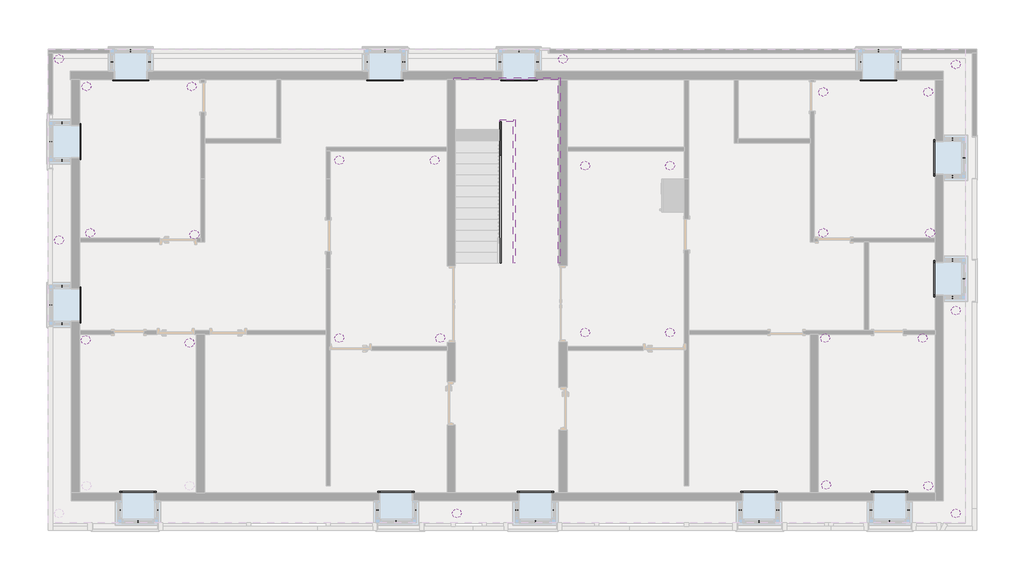
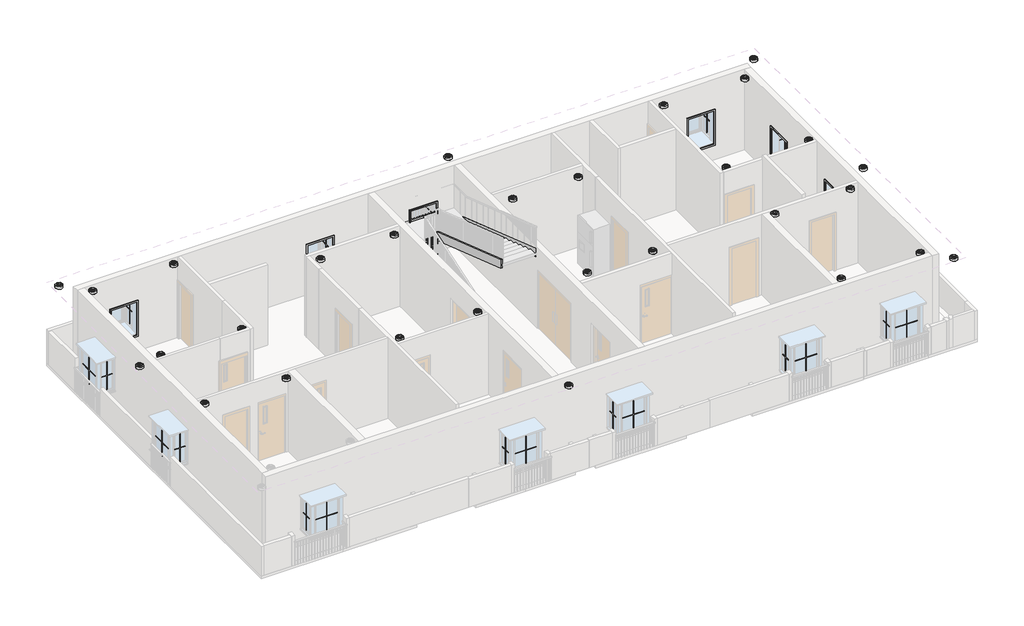
# One storey, part 7 of 7: 52 proxies, 29 light fixtures, 6 members.
"""IFC4 building model written with IfcOpenShell, lengths in millimetres."""

from ifc_helpers import new_model, si_unit, frame, origin, place, context, project, spatial, polyline, outline, extrude, transform, mapped, element, save
from components import muntin_pattern_2x2_muntin_pattern_2x2_95b57395, muntin_pattern_2x2_muntin_pattern_2x2_f03ab90d, trim_window_interior_flat_picture_frame_e50cf7ae, ceiling_light_flat_round_60w_120v_7c4c2a52

model = new_model("IFC4")

# Units and contexts
model_context = context("Model", 3, world=origin())
ifc_project = project(units=[si_unit("LENGTHUNIT", "METRE", prefix="MILLI")], contexts=[model_context])

# Site, building, storey
site = spatial("IfcSite", under=ifc_project)
building = spatial("IfcBuilding", under=site)
storey = spatial("IfcBuildingStorey", under=building, Elevation=3200.4)

# Proxies
placement = place(None, origin())
muntin_pattern_2x2_muntin_pattern_2x2_shape = muntin_pattern_2x2_muntin_pattern_2x2_95b57395(model_context)
element("IfcBuildingElementProxy", 1, Name="Muntin Pattern_2x2 : Muntin Pattern_2x2", ObjectType="Muntin Pattern_2x2 : Muntin Pattern_2x2", at=placement, inside=storey, context=model_context, shape_type="MappedRepresentation", body=[
    mapped(muntin_pattern_2x2_muntin_pattern_2x2_shape, transform((-10814.9987925, 8428.7317329, 3930.65), x_axis=(1.0, 0.0, 0.0), y_axis=(0.0, 1.0, 0.0), z_axis=(0.0, 0.0, 1.0))),
])
element("IfcBuildingElementProxy", 2, Name="Muntin Pattern_2x2 : Muntin Pattern_2x2", ObjectType="Muntin Pattern_2x2 : Muntin Pattern_2x2", at=placement, inside=storey, context=model_context, shape_type="MappedRepresentation", body=[
    mapped(muntin_pattern_2x2_muntin_pattern_2x2_shape, transform((-3791.8987998, 8428.7317329, 3930.65), x_axis=(1.0, 0.0, 0.0), y_axis=(0.0, 1.0, 0.0), z_axis=(0.0, 0.0, 1.0))),
])
element("IfcBuildingElementProxy", 3, Name="Muntin Pattern_2x2 : Muntin Pattern_2x2", ObjectType="Muntin Pattern_2x2 : Muntin Pattern_2x2", at=placement, inside=storey, context=model_context, shape_type="MappedRepresentation", body=[
    mapped(muntin_pattern_2x2_muntin_pattern_2x2_shape, transform((-96.7067989, 8428.7317329, 3930.65), x_axis=(1.0, 0.0, 0.0), y_axis=(0.0, 1.0, 0.0), z_axis=(0.0, 0.0, 1.0))),
])
element("IfcBuildingElementProxy", 4, Name="Muntin Pattern_2x2 : Muntin Pattern_2x2", ObjectType="Muntin Pattern_2x2 : Muntin Pattern_2x2", at=placement, inside=storey, context=model_context, shape_type="MappedRepresentation", body=[
    mapped(muntin_pattern_2x2_muntin_pattern_2x2_shape, transform((9835.2012075, 8428.7317329, 3930.65), x_axis=(1.0, 0.0, 0.0), y_axis=(0.0, 1.0, 0.0), z_axis=(0.0, 0.0, 1.0))),
])
element("IfcBuildingElementProxy", 5, Name="Muntin Pattern_2x2 : Muntin Pattern_2x2", ObjectType="Muntin Pattern_2x2 : Muntin Pattern_2x2", at=placement, inside=storey, context=model_context, shape_type="MappedRepresentation", body=[
    mapped(muntin_pattern_2x2_muntin_pattern_2x2_shape, transform((-10611.7987958, -4582.4182193, 3930.65), x_axis=(-1.0, 0.0, 0.0), y_axis=(0.0, -1.0, 0.0), z_axis=(0.0, 0.0, 1.0))),
])
element("IfcBuildingElementProxy", 6, Name="Muntin Pattern_2x2 : Muntin Pattern_2x2", ObjectType="Muntin Pattern_2x2 : Muntin Pattern_2x2", at=placement, inside=storey, context=model_context, shape_type="MappedRepresentation", body=[
    mapped(muntin_pattern_2x2_muntin_pattern_2x2_shape, transform((-3487.0987998, -4582.4182193, 3930.65), x_axis=(-1.0, 0.0, 0.0), y_axis=(0.0, -1.0, 0.0), z_axis=(0.0, 0.0, 1.0))),
])
element("IfcBuildingElementProxy", 7, Name="Muntin Pattern_2x2 : Muntin Pattern_2x2", ObjectType="Muntin Pattern_2x2 : Muntin Pattern_2x2", at=placement, inside=storey, context=model_context, shape_type="MappedRepresentation", body=[
    mapped(muntin_pattern_2x2_muntin_pattern_2x2_shape, transform((360.4932011, -4582.4182193, 3930.65), x_axis=(-1.0, 0.0, 0.0), y_axis=(0.0, -1.0, 0.0), z_axis=(0.0, 0.0, 1.0))),
])
element("IfcBuildingElementProxy", 8, Name="Muntin Pattern_2x2 : Muntin Pattern_2x2", ObjectType="Muntin Pattern_2x2 : Muntin Pattern_2x2", at=placement, inside=storey, context=model_context, shape_type="MappedRepresentation", body=[
    mapped(muntin_pattern_2x2_muntin_pattern_2x2_shape, transform((6533.2012079, -4582.4182193, 3930.65), x_axis=(-1.0, 0.0, 0.0), y_axis=(0.0, -1.0, 0.0), z_axis=(0.0, 0.0, 1.0))),
])
element("IfcBuildingElementProxy", 9, Name="Muntin Pattern_2x2 : Muntin Pattern_2x2", ObjectType="Muntin Pattern_2x2 : Muntin Pattern_2x2", at=placement, inside=storey, context=model_context, shape_type="MappedRepresentation", body=[
    mapped(muntin_pattern_2x2_muntin_pattern_2x2_shape, transform((10140.0012075, -4582.4182193, 3930.65), x_axis=(-1.0, 0.0, 0.0), y_axis=(0.0, -1.0, 0.0), z_axis=(0.0, 0.0, 1.0))),
])
element("IfcBuildingElementProxy", 10, Name="Muntin Pattern_2x2 : Muntin Pattern_2x2", ObjectType="Muntin Pattern_2x2 : Muntin Pattern_2x2", at=placement, inside=storey, context=model_context, shape_type="MappedRepresentation", body=[
    mapped(muntin_pattern_2x2_muntin_pattern_2x2_shape, transform((12194.2262075, 2126.3567332, 3930.65), x_axis=(0.0, -1.0, 0.0), y_axis=(1.0, 0.0, 0.0), z_axis=(0.0, 0.0, 1.0))),
])
element("IfcBuildingElementProxy", 11, Name="Muntin Pattern_2x2 : Muntin Pattern_2x2", ObjectType="Muntin Pattern_2x2 : Muntin Pattern_2x2", at=placement, inside=storey, context=model_context, shape_type="MappedRepresentation", body=[
    mapped(muntin_pattern_2x2_muntin_pattern_2x2_shape, transform((12194.2262075, 5469.631733, 3930.65), x_axis=(0.0, -1.0, 0.0), y_axis=(1.0, 0.0, 0.0), z_axis=(0.0, 0.0, 1.0))),
])
element("IfcBuildingElementProxy", 12, Name="Muntin Pattern_2x2 : Muntin Pattern_2x2", ObjectType="Muntin Pattern_2x2 : Muntin Pattern_2x2", at=placement, inside=storey, context=model_context, shape_type="MappedRepresentation", body=[
    mapped(muntin_pattern_2x2_muntin_pattern_2x2_shape, transform((-13021.6237925, 1402.4567334, 3930.65), x_axis=(0.0, 1.0, 0.0), y_axis=(-1.0, 0.0, 0.0), z_axis=(0.0, 0.0, 1.0))),
])
element("IfcBuildingElementProxy", 13, Name="Muntin Pattern_2x2 : Muntin Pattern_2x2", ObjectType="Muntin Pattern_2x2 : Muntin Pattern_2x2", at=placement, inside=storey, context=model_context, shape_type="MappedRepresentation", body=[
    mapped(muntin_pattern_2x2_muntin_pattern_2x2_shape, transform((-13021.6237925, 5917.3067329, 3930.65), x_axis=(0.0, 1.0, 0.0), y_axis=(-1.0, 0.0, 0.0), z_axis=(0.0, 0.0, 1.0))),
])
muntin_pattern_2x2_muntin_pattern_2x2_2_shape = muntin_pattern_2x2_muntin_pattern_2x2_f03ab90d(model_context)
element("IfcBuildingElementProxy", 14, Name="Muntin Pattern_2x2 : Muntin Pattern_2x2", ObjectType="Muntin Pattern_2x2 : Muntin Pattern_2x2", at=placement, inside=storey, context=model_context, shape_type="MappedRepresentation", body=[
    mapped(muntin_pattern_2x2_muntin_pattern_2x2_2_shape, transform((-11332.5237925, 8114.4067329, 3930.65), x_axis=(0.0, -1.0, 0.0), y_axis=(1.0, 0.0, 0.0), z_axis=(0.0, 0.0, 1.0))),
])
element("IfcBuildingElementProxy", 15, Name="Muntin Pattern_2x2 : Muntin Pattern_2x2", ObjectType="Muntin Pattern_2x2 : Muntin Pattern_2x2", at=placement, inside=storey, context=model_context, shape_type="MappedRepresentation", body=[
    mapped(muntin_pattern_2x2_muntin_pattern_2x2_2_shape, transform((-10297.4737925, 8114.4067329, 3930.65), x_axis=(0.0, 1.0, 0.0), y_axis=(-1.0, 0.0, 0.0), z_axis=(0.0, 0.0, 1.0))),
])
element("IfcBuildingElementProxy", 16, Name="Muntin Pattern_2x2 : Muntin Pattern_2x2", ObjectType="Muntin Pattern_2x2 : Muntin Pattern_2x2", at=placement, inside=storey, context=model_context, shape_type="MappedRepresentation", body=[
    mapped(muntin_pattern_2x2_muntin_pattern_2x2_2_shape, transform((-4309.4237998, 8114.4067329, 3930.65), x_axis=(0.0, -1.0, 0.0), y_axis=(1.0, 0.0, 0.0), z_axis=(0.0, 0.0, 1.0))),
])
element("IfcBuildingElementProxy", 17, Name="Muntin Pattern_2x2 : Muntin Pattern_2x2", ObjectType="Muntin Pattern_2x2 : Muntin Pattern_2x2", at=placement, inside=storey, context=model_context, shape_type="MappedRepresentation", body=[
    mapped(muntin_pattern_2x2_muntin_pattern_2x2_2_shape, transform((-3274.3737998, 8114.4067329, 3930.65), x_axis=(0.0, 1.0, 0.0), y_axis=(-1.0, 0.0, 0.0), z_axis=(0.0, 0.0, 1.0))),
])
element("IfcBuildingElementProxy", 18, Name="Muntin Pattern_2x2 : Muntin Pattern_2x2", ObjectType="Muntin Pattern_2x2 : Muntin Pattern_2x2", at=placement, inside=storey, context=model_context, shape_type="MappedRepresentation", body=[
    mapped(muntin_pattern_2x2_muntin_pattern_2x2_2_shape, transform((-614.2317989, 8114.4067329, 3930.65), x_axis=(0.0, -1.0, 0.0), y_axis=(1.0, 0.0, 0.0), z_axis=(0.0, 0.0, 1.0))),
])
element("IfcBuildingElementProxy", 19, Name="Muntin Pattern_2x2 : Muntin Pattern_2x2", ObjectType="Muntin Pattern_2x2 : Muntin Pattern_2x2", at=placement, inside=storey, context=model_context, shape_type="MappedRepresentation", body=[
    mapped(muntin_pattern_2x2_muntin_pattern_2x2_2_shape, transform((420.8182011, 8114.4067329, 3930.65), x_axis=(0.0, 1.0, 0.0), y_axis=(-1.0, 0.0, 0.0), z_axis=(0.0, 0.0, 1.0))),
])
element("IfcBuildingElementProxy", 20, Name="Muntin Pattern_2x2 : Muntin Pattern_2x2", ObjectType="Muntin Pattern_2x2 : Muntin Pattern_2x2", at=placement, inside=storey, context=model_context, shape_type="MappedRepresentation", body=[
    mapped(muntin_pattern_2x2_muntin_pattern_2x2_2_shape, transform((9317.6762075, 8114.4067329, 3930.65), x_axis=(0.0, -1.0, 0.0), y_axis=(1.0, 0.0, 0.0), z_axis=(0.0, 0.0, 1.0))),
])
element("IfcBuildingElementProxy", 21, Name="Muntin Pattern_2x2 : Muntin Pattern_2x2", ObjectType="Muntin Pattern_2x2 : Muntin Pattern_2x2", at=placement, inside=storey, context=model_context, shape_type="MappedRepresentation", body=[
    mapped(muntin_pattern_2x2_muntin_pattern_2x2_2_shape, transform((10352.7262075, 8114.4067329, 3930.65), x_axis=(0.0, 1.0, 0.0), y_axis=(-1.0, 0.0, 0.0), z_axis=(0.0, 0.0, 1.0))),
])
element("IfcBuildingElementProxy", 22, Name="Muntin Pattern_2x2 : Muntin Pattern_2x2", ObjectType="Muntin Pattern_2x2 : Muntin Pattern_2x2", at=placement, inside=storey, context=model_context, shape_type="MappedRepresentation", body=[
    mapped(muntin_pattern_2x2_muntin_pattern_2x2_2_shape, transform((-10094.2737958, -4268.0932193, 3930.65), x_axis=(0.0, 1.0, 0.0), y_axis=(-1.0, 0.0, 0.0), z_axis=(0.0, 0.0, 1.0))),
])
element("IfcBuildingElementProxy", 23, Name="Muntin Pattern_2x2 : Muntin Pattern_2x2", ObjectType="Muntin Pattern_2x2 : Muntin Pattern_2x2", at=placement, inside=storey, context=model_context, shape_type="MappedRepresentation", body=[
    mapped(muntin_pattern_2x2_muntin_pattern_2x2_2_shape, transform((-11129.3237958, -4268.0932193, 3930.65), x_axis=(0.0, -1.0, 0.0), y_axis=(1.0, 0.0, 0.0), z_axis=(0.0, 0.0, 1.0))),
])
element("IfcBuildingElementProxy", 24, Name="Muntin Pattern_2x2 : Muntin Pattern_2x2", ObjectType="Muntin Pattern_2x2 : Muntin Pattern_2x2", at=placement, inside=storey, context=model_context, shape_type="MappedRepresentation", body=[
    mapped(muntin_pattern_2x2_muntin_pattern_2x2_2_shape, transform((-2969.5737998, -4268.0932193, 3930.65), x_axis=(0.0, 1.0, 0.0), y_axis=(-1.0, 0.0, 0.0), z_axis=(0.0, 0.0, 1.0))),
])
element("IfcBuildingElementProxy", 25, Name="Muntin Pattern_2x2 : Muntin Pattern_2x2", ObjectType="Muntin Pattern_2x2 : Muntin Pattern_2x2", at=placement, inside=storey, context=model_context, shape_type="MappedRepresentation", body=[
    mapped(muntin_pattern_2x2_muntin_pattern_2x2_2_shape, transform((-4004.6237998, -4268.0932193, 3930.65), x_axis=(0.0, -1.0, 0.0), y_axis=(1.0, 0.0, 0.0), z_axis=(0.0, 0.0, 1.0))),
])
element("IfcBuildingElementProxy", 26, Name="Muntin Pattern_2x2 : Muntin Pattern_2x2", ObjectType="Muntin Pattern_2x2 : Muntin Pattern_2x2", at=placement, inside=storey, context=model_context, shape_type="MappedRepresentation", body=[
    mapped(muntin_pattern_2x2_muntin_pattern_2x2_2_shape, transform((878.0182011, -4268.0932193, 3930.65), x_axis=(0.0, 1.0, 0.0), y_axis=(-1.0, 0.0, 0.0), z_axis=(0.0, 0.0, 1.0))),
])
element("IfcBuildingElementProxy", 27, Name="Muntin Pattern_2x2 : Muntin Pattern_2x2", ObjectType="Muntin Pattern_2x2 : Muntin Pattern_2x2", at=placement, inside=storey, context=model_context, shape_type="MappedRepresentation", body=[
    mapped(muntin_pattern_2x2_muntin_pattern_2x2_2_shape, transform((-157.0317989, -4268.0932193, 3930.65), x_axis=(0.0, -1.0, 0.0), y_axis=(1.0, 0.0, 0.0), z_axis=(0.0, 0.0, 1.0))),
])
element("IfcBuildingElementProxy", 28, Name="Muntin Pattern_2x2 : Muntin Pattern_2x2", ObjectType="Muntin Pattern_2x2 : Muntin Pattern_2x2", at=placement, inside=storey, context=model_context, shape_type="MappedRepresentation", body=[
    mapped(muntin_pattern_2x2_muntin_pattern_2x2_2_shape, transform((7050.7262079, -4268.0932193, 3930.65), x_axis=(0.0, 1.0, 0.0), y_axis=(-1.0, 0.0, 0.0), z_axis=(0.0, 0.0, 1.0))),
])
element("IfcBuildingElementProxy", 29, Name="Muntin Pattern_2x2 : Muntin Pattern_2x2", ObjectType="Muntin Pattern_2x2 : Muntin Pattern_2x2", at=placement, inside=storey, context=model_context, shape_type="MappedRepresentation", body=[
    mapped(muntin_pattern_2x2_muntin_pattern_2x2_2_shape, transform((6015.6762079, -4268.0932193, 3930.65), x_axis=(0.0, -1.0, 0.0), y_axis=(1.0, 0.0, 0.0), z_axis=(0.0, 0.0, 1.0))),
])
element("IfcBuildingElementProxy", 30, Name="Muntin Pattern_2x2 : Muntin Pattern_2x2", ObjectType="Muntin Pattern_2x2 : Muntin Pattern_2x2", at=placement, inside=storey, context=model_context, shape_type="MappedRepresentation", body=[
    mapped(muntin_pattern_2x2_muntin_pattern_2x2_2_shape, transform((10657.5262075, -4268.0932193, 3930.65), x_axis=(0.0, 1.0, 0.0), y_axis=(-1.0, 0.0, 0.0), z_axis=(0.0, 0.0, 1.0))),
])
element("IfcBuildingElementProxy", 31, Name="Muntin Pattern_2x2 : Muntin Pattern_2x2", ObjectType="Muntin Pattern_2x2 : Muntin Pattern_2x2", at=placement, inside=storey, context=model_context, shape_type="MappedRepresentation", body=[
    mapped(muntin_pattern_2x2_muntin_pattern_2x2_2_shape, transform((9622.4762075, -4268.0932193, 3930.65), x_axis=(0.0, -1.0, 0.0), y_axis=(1.0, 0.0, 0.0), z_axis=(0.0, 0.0, 1.0))),
])
element("IfcBuildingElementProxy", 32, Name="Muntin Pattern_2x2 : Muntin Pattern_2x2", ObjectType="Muntin Pattern_2x2 : Muntin Pattern_2x2", at=placement, inside=storey, context=model_context, shape_type="MappedRepresentation", body=[
    mapped(muntin_pattern_2x2_muntin_pattern_2x2_2_shape, transform((11879.9012075, 2643.8817332, 3930.65), x_axis=(-1.0, 0.0, 0.0), y_axis=(0.0, -1.0, 0.0), z_axis=(0.0, 0.0, 1.0))),
])
element("IfcBuildingElementProxy", 33, Name="Muntin Pattern_2x2 : Muntin Pattern_2x2", ObjectType="Muntin Pattern_2x2 : Muntin Pattern_2x2", at=placement, inside=storey, context=model_context, shape_type="MappedRepresentation", body=[
    mapped(muntin_pattern_2x2_muntin_pattern_2x2_2_shape, transform((11879.9012075, 1608.8317332, 3930.65), x_axis=(1.0, 0.0, 0.0), y_axis=(0.0, 1.0, 0.0), z_axis=(0.0, 0.0, 1.0))),
])
element("IfcBuildingElementProxy", 34, Name="Muntin Pattern_2x2 : Muntin Pattern_2x2", ObjectType="Muntin Pattern_2x2 : Muntin Pattern_2x2", at=placement, inside=storey, context=model_context, shape_type="MappedRepresentation", body=[
    mapped(muntin_pattern_2x2_muntin_pattern_2x2_2_shape, transform((11879.9012075, 5987.156733, 3930.65), x_axis=(-1.0, 0.0, 0.0), y_axis=(0.0, -1.0, 0.0), z_axis=(0.0, 0.0, 1.0))),
])
element("IfcBuildingElementProxy", 35, Name="Muntin Pattern_2x2 : Muntin Pattern_2x2", ObjectType="Muntin Pattern_2x2 : Muntin Pattern_2x2", at=placement, inside=storey, context=model_context, shape_type="MappedRepresentation", body=[
    mapped(muntin_pattern_2x2_muntin_pattern_2x2_2_shape, transform((11879.9012075, 4952.106733, 3930.65), x_axis=(1.0, 0.0, 0.0), y_axis=(0.0, 1.0, 0.0), z_axis=(0.0, 0.0, 1.0))),
])
element("IfcBuildingElementProxy", 36, Name="Muntin Pattern_2x2 : Muntin Pattern_2x2", ObjectType="Muntin Pattern_2x2 : Muntin Pattern_2x2", at=placement, inside=storey, context=model_context, shape_type="MappedRepresentation", body=[
    mapped(muntin_pattern_2x2_muntin_pattern_2x2_2_shape, transform((-12707.2987925, 884.9317334, 3930.65), x_axis=(1.0, 0.0, 0.0), y_axis=(0.0, 1.0, 0.0), z_axis=(0.0, 0.0, 1.0))),
])
element("IfcBuildingElementProxy", 37, Name="Muntin Pattern_2x2 : Muntin Pattern_2x2", ObjectType="Muntin Pattern_2x2 : Muntin Pattern_2x2", at=placement, inside=storey, context=model_context, shape_type="MappedRepresentation", body=[
    mapped(muntin_pattern_2x2_muntin_pattern_2x2_2_shape, transform((-12707.2987925, 1919.9817334, 3930.65), x_axis=(-1.0, 0.0, 0.0), y_axis=(0.0, -1.0, 0.0), z_axis=(0.0, 0.0, 1.0))),
])
element("IfcBuildingElementProxy", 38, Name="Muntin Pattern_2x2 : Muntin Pattern_2x2", ObjectType="Muntin Pattern_2x2 : Muntin Pattern_2x2", at=placement, inside=storey, context=model_context, shape_type="MappedRepresentation", body=[
    mapped(muntin_pattern_2x2_muntin_pattern_2x2_2_shape, transform((-12707.2987925, 5399.7817329, 3930.65), x_axis=(1.0, 0.0, 0.0), y_axis=(0.0, 1.0, 0.0), z_axis=(0.0, 0.0, 1.0))),
])
element("IfcBuildingElementProxy", 39, Name="Muntin Pattern_2x2 : Muntin Pattern_2x2", ObjectType="Muntin Pattern_2x2 : Muntin Pattern_2x2", at=placement, inside=storey, context=model_context, shape_type="MappedRepresentation", body=[
    mapped(muntin_pattern_2x2_muntin_pattern_2x2_2_shape, transform((-12707.2987925, 6434.8317329, 3930.65), x_axis=(-1.0, 0.0, 0.0), y_axis=(0.0, -1.0, 0.0), z_axis=(0.0, 0.0, 1.0))),
])
trim_window_interior_flat_picture_frame_shape = trim_window_interior_flat_picture_frame_e50cf7ae(model_context)
element("IfcBuildingElementProxy", 40, Name="Trim-Window-Interior-Flat : Picture Frame", ObjectType="Trim-Window-Interior-Flat : Picture Frame", at=placement, inside=storey, context=model_context, shape_type="MappedRepresentation", body=[
    mapped(trim_window_interior_flat_picture_frame_shape, transform((-10814.9987925, 7631.8067329, 5080.0), x_axis=(1.0, 0.0, 0.0), y_axis=(0.0, 0.0, 1.0), z_axis=(0.0, -1.0, 0.0))),
])
element("IfcBuildingElementProxy", 41, Name="Trim-Window-Interior-Flat : Picture Frame", ObjectType="Trim-Window-Interior-Flat : Picture Frame", at=placement, inside=storey, context=model_context, shape_type="MappedRepresentation", body=[
    mapped(trim_window_interior_flat_picture_frame_shape, transform((-3791.8987998, 7631.8067329, 5080.0), x_axis=(1.0, 0.0, 0.0), y_axis=(0.0, 0.0, 1.0), z_axis=(0.0, -1.0, 0.0))),
])
element("IfcBuildingElementProxy", 42, Name="Trim-Window-Interior-Flat : Picture Frame", ObjectType="Trim-Window-Interior-Flat : Picture Frame", at=placement, inside=storey, context=model_context, shape_type="MappedRepresentation", body=[
    mapped(trim_window_interior_flat_picture_frame_shape, transform((-96.7067989, 7631.8067329, 5080.0), x_axis=(1.0, 0.0, 0.0), y_axis=(0.0, 0.0, 1.0), z_axis=(0.0, -1.0, 0.0))),
])
element("IfcBuildingElementProxy", 43, Name="Trim-Window-Interior-Flat : Picture Frame", ObjectType="Trim-Window-Interior-Flat : Picture Frame", at=placement, inside=storey, context=model_context, shape_type="MappedRepresentation", body=[
    mapped(trim_window_interior_flat_picture_frame_shape, transform((9835.2012075, 7631.8067329, 5080.0), x_axis=(1.0, 0.0, 0.0), y_axis=(0.0, 0.0, 1.0), z_axis=(0.0, -1.0, 0.0))),
])
element("IfcBuildingElementProxy", 44, Name="Trim-Window-Interior-Flat : Picture Frame", ObjectType="Trim-Window-Interior-Flat : Picture Frame", at=placement, inside=storey, context=model_context, shape_type="MappedRepresentation", body=[
    mapped(trim_window_interior_flat_picture_frame_shape, transform((-10611.7987958, -3785.4932193, 5080.0), x_axis=(-1.0, 0.0, 0.0), y_axis=(0.0, 0.0, 1.0), z_axis=(0.0, 1.0, 0.0))),
])
element("IfcBuildingElementProxy", 45, Name="Trim-Window-Interior-Flat : Picture Frame", ObjectType="Trim-Window-Interior-Flat : Picture Frame", at=placement, inside=storey, context=model_context, shape_type="MappedRepresentation", body=[
    mapped(trim_window_interior_flat_picture_frame_shape, transform((-3487.0987998, -3785.4932193, 5080.0), x_axis=(-1.0, 0.0, 0.0), y_axis=(0.0, 0.0, 1.0), z_axis=(0.0, 1.0, 0.0))),
])
element("IfcBuildingElementProxy", 46, Name="Trim-Window-Interior-Flat : Picture Frame", ObjectType="Trim-Window-Interior-Flat : Picture Frame", at=placement, inside=storey, context=model_context, shape_type="MappedRepresentation", body=[
    mapped(trim_window_interior_flat_picture_frame_shape, transform((360.4932011, -3785.4932193, 5080.0), x_axis=(-1.0, 0.0, 0.0), y_axis=(0.0, 0.0, 1.0), z_axis=(0.0, 1.0, 0.0))),
])
element("IfcBuildingElementProxy", 47, Name="Trim-Window-Interior-Flat : Picture Frame", ObjectType="Trim-Window-Interior-Flat : Picture Frame", at=placement, inside=storey, context=model_context, shape_type="MappedRepresentation", body=[
    mapped(trim_window_interior_flat_picture_frame_shape, transform((6533.2012079, -3785.4932193, 5080.0), x_axis=(-1.0, 0.0, 0.0), y_axis=(0.0, 0.0, 1.0), z_axis=(0.0, 1.0, 0.0))),
])
element("IfcBuildingElementProxy", 48, Name="Trim-Window-Interior-Flat : Picture Frame", ObjectType="Trim-Window-Interior-Flat : Picture Frame", at=placement, inside=storey, context=model_context, shape_type="MappedRepresentation", body=[
    mapped(trim_window_interior_flat_picture_frame_shape, transform((10140.0012075, -3785.4932193, 5080.0), x_axis=(-1.0, 0.0, 0.0), y_axis=(0.0, 0.0, 1.0), z_axis=(0.0, 1.0, 0.0))),
])
element("IfcBuildingElementProxy", 49, Name="Trim-Window-Interior-Flat : Picture Frame", ObjectType="Trim-Window-Interior-Flat : Picture Frame", at=placement, inside=storey, context=model_context, shape_type="MappedRepresentation", body=[
    mapped(trim_window_interior_flat_picture_frame_shape, transform((11397.3012075, 2126.3567332, 5080.0), x_axis=(0.0, -1.0, 0.0), y_axis=(0.0, 0.0, 1.0), z_axis=(-1.0, 0.0, 0.0))),
])
element("IfcBuildingElementProxy", 50, Name="Trim-Window-Interior-Flat : Picture Frame", ObjectType="Trim-Window-Interior-Flat : Picture Frame", at=placement, inside=storey, context=model_context, shape_type="MappedRepresentation", body=[
    mapped(trim_window_interior_flat_picture_frame_shape, transform((11397.3012075, 5469.631733, 5080.0), x_axis=(0.0, -1.0, 0.0), y_axis=(0.0, 0.0, 1.0), z_axis=(-1.0, 0.0, 0.0))),
])
element("IfcBuildingElementProxy", 51, Name="Trim-Window-Interior-Flat : Picture Frame", ObjectType="Trim-Window-Interior-Flat : Picture Frame", at=placement, inside=storey, context=model_context, shape_type="MappedRepresentation", body=[
    mapped(trim_window_interior_flat_picture_frame_shape, transform((-12224.6987925, 1402.4567334, 5080.0), x_axis=(0.0, 1.0, 0.0), y_axis=(0.0, 0.0, 1.0), z_axis=(1.0, 0.0, 0.0))),
])
element("IfcBuildingElementProxy", 52, Name="Trim-Window-Interior-Flat : Picture Frame", ObjectType="Trim-Window-Interior-Flat : Picture Frame", at=placement, inside=storey, context=model_context, shape_type="MappedRepresentation", body=[
    mapped(trim_window_interior_flat_picture_frame_shape, transform((-12224.6987925, 5917.3067329, 5080.0), x_axis=(0.0, 1.0, 0.0), y_axis=(0.0, 0.0, 1.0), z_axis=(1.0, 0.0, 0.0))),
])

# Light fixtures
ceiling_light_flat_round_60w_120v_shape = ceiling_light_flat_round_60w_120v_7c4c2a52(model_context)
element("IfcLightFixture", 53, ObjectType="Ceiling Light - Flat Round : 60W - 120V", at=placement, inside=storey, context=model_context, shape_type="MappedRepresentation", body=[
    mapped(ceiling_light_flat_round_60w_120v_shape, transform((-12796.1987925, 8203.3067329, 3810.0), x_axis=(1.0, 0.0, 0.0), y_axis=(0.0, 1.0, 0.0), z_axis=(0.0, 0.0, 1.0))),
])
element("IfcLightFixture", 54, ObjectType="Ceiling Light - Flat Round : 60W - 120V", at=placement, inside=storey, context=model_context, shape_type="MappedRepresentation", body=[
    mapped(ceiling_light_flat_round_60w_120v_shape, transform((-12796.1987925, 3193.1567332, 3810.0), x_axis=(1.0, 0.0, 0.0), y_axis=(0.0, 1.0, 0.0), z_axis=(0.0, 0.0, 1.0))),
])
element("IfcLightFixture", 55, ObjectType="Ceiling Light - Flat Round : 60W - 120V", at=placement, inside=storey, context=model_context, shape_type="MappedRepresentation", body=[
    mapped(ceiling_light_flat_round_60w_120v_shape, transform((-1810.6987998, -4356.9932193, 3810.0), x_axis=(1.0, 0.0, 0.0), y_axis=(0.0, 1.0, 0.0), z_axis=(0.0, 0.0, 1.0))),
])
element("IfcLightFixture", 56, ObjectType="Ceiling Light - Flat Round : 60W - 120V", at=placement, inside=storey, context=model_context, shape_type="MappedRepresentation", body=[
    mapped(ceiling_light_flat_round_60w_120v_shape, transform((11968.8012075, -4356.9932193, 3810.0), x_axis=(1.0, 0.0, 0.0), y_axis=(0.0, 1.0, 0.0), z_axis=(0.0, 0.0, 1.0))),
])
element("IfcLightFixture", 57, ObjectType="Ceiling Light - Flat Round : 60W - 120V", at=placement, inside=storey, context=model_context, shape_type="MappedRepresentation", body=[
    mapped(ceiling_light_flat_round_60w_120v_shape, transform((11968.8012075, 1250.0567334, 3810.0), x_axis=(1.0, 0.0, 0.0), y_axis=(0.0, 1.0, 0.0), z_axis=(0.0, 0.0, 1.0))),
])
element("IfcLightFixture", 58, ObjectType="Ceiling Light - Flat Round : 60W - 120V", at=placement, inside=storey, context=model_context, shape_type="MappedRepresentation", body=[
    mapped(ceiling_light_flat_round_60w_120v_shape, transform((11968.8012075, 8050.9067329, 3810.0), x_axis=(1.0, 0.0, 0.0), y_axis=(0.0, 1.0, 0.0), z_axis=(0.0, 0.0, 1.0))),
])
element("IfcLightFixture", 59, ObjectType="Ceiling Light - Flat Round : 60W - 120V", at=placement, inside=storey, context=model_context, shape_type="MappedRepresentation", body=[
    mapped(ceiling_light_flat_round_60w_120v_shape, transform((1122.4932011, 8203.3067329, 3810.0), x_axis=(1.0, 0.0, 0.0), y_axis=(0.0, 1.0, 0.0), z_axis=(0.0, 0.0, 1.0))),
])
element("IfcLightFixture", 60, ObjectType="Ceiling Light - Flat Round : 60W - 120V", at=placement, inside=storey, context=model_context, shape_type="MappedRepresentation", body=[
    mapped(ceiling_light_flat_round_60w_120v_shape, transform((-9189.3987992, 357.6578621, 3810.0), x_axis=(1.0, 0.0, 0.0), y_axis=(0.0, 1.0, 0.0), z_axis=(0.0, 0.0, 1.0))),
])
element("IfcLightFixture", 61, ObjectType="Ceiling Light - Flat Round : 60W - 120V", at=placement, inside=storey, context=model_context, shape_type="MappedRepresentation", body=[
    mapped(ceiling_light_flat_round_60w_120v_shape, transform((-12059.5987925, 437.2567334, 3810.0), x_axis=(1.0, 0.0, 0.0), y_axis=(0.0, 1.0, 0.0), z_axis=(0.0, 0.0, 1.0))),
])
element("IfcLightFixture", 62, ObjectType="Ceiling Light - Flat Round : 60W - 120V", at=placement, inside=storey, context=model_context, shape_type="MappedRepresentation", body=[
    mapped(ceiling_light_flat_round_60w_120v_shape, transform((-12034.1987925, 7441.3067329, 3810.0), x_axis=(1.0, 0.0, 0.0), y_axis=(0.0, 1.0, 0.0), z_axis=(0.0, 0.0, 1.0))),
])
element("IfcLightFixture", 63, ObjectType="Ceiling Light - Flat Round : 60W - 120V", at=placement, inside=storey, context=model_context, shape_type="MappedRepresentation", body=[
    mapped(ceiling_light_flat_round_60w_120v_shape, transform((-9132.2487992, 7441.3067329, 3810.0), x_axis=(1.0, 0.0, 0.0), y_axis=(0.0, 1.0, 0.0), z_axis=(0.0, 0.0, 1.0))),
])
element("IfcLightFixture", 64, ObjectType="Ceiling Light - Flat Round : 60W - 120V", at=placement, inside=storey, context=model_context, shape_type="MappedRepresentation", body=[
    mapped(ceiling_light_flat_round_60w_120v_shape, transform((-11932.5987925, 3396.3567332, 3810.0), x_axis=(1.0, 0.0, 0.0), y_axis=(0.0, 1.0, 0.0), z_axis=(0.0, 0.0, 1.0))),
])
element("IfcLightFixture", 65, ObjectType="Ceiling Light - Flat Round : 60W - 120V", at=placement, inside=storey, context=model_context, shape_type="MappedRepresentation", body=[
    mapped(ceiling_light_flat_round_60w_120v_shape, transform((-9056.0487992, 3345.5567332, 3810.0), x_axis=(1.0, 0.0, 0.0), y_axis=(0.0, 1.0, 0.0), z_axis=(0.0, 0.0, 1.0))),
])
element("IfcLightFixture", 66, ObjectType="Ceiling Light - Flat Round : 60W - 120V", at=placement, inside=storey, context=model_context, shape_type="MappedRepresentation", body=[
    mapped(ceiling_light_flat_round_60w_120v_shape, transform((8304.8512079, 7288.9067329, 3810.0), x_axis=(1.0, 0.0, 0.0), y_axis=(0.0, 1.0, 0.0), z_axis=(0.0, 0.0, 1.0))),
])
element("IfcLightFixture", 67, ObjectType="Ceiling Light - Flat Round : 60W - 120V", at=placement, inside=storey, context=model_context, shape_type="MappedRepresentation", body=[
    mapped(ceiling_light_flat_round_60w_120v_shape, transform((11206.8012075, 7288.9067329, 3810.0), x_axis=(1.0, 0.0, 0.0), y_axis=(0.0, 1.0, 0.0), z_axis=(0.0, 0.0, 1.0))),
])
element("IfcLightFixture", 68, ObjectType="Ceiling Light - Flat Round : 60W - 120V", at=placement, inside=storey, context=model_context, shape_type="MappedRepresentation", body=[
    mapped(ceiling_light_flat_round_60w_120v_shape, transform((8304.8512079, 3396.3567332, 3810.0), x_axis=(1.0, 0.0, 0.0), y_axis=(0.0, 1.0, 0.0), z_axis=(0.0, 0.0, 1.0))),
])
element("IfcLightFixture", 69, ObjectType="Ceiling Light - Flat Round : 60W - 120V", at=placement, inside=storey, context=model_context, shape_type="MappedRepresentation", body=[
    mapped(ceiling_light_flat_round_60w_120v_shape, transform((11257.6012075, 3396.3567332, 3810.0), x_axis=(1.0, 0.0, 0.0), y_axis=(0.0, 1.0, 0.0), z_axis=(0.0, 0.0, 1.0))),
])
element("IfcLightFixture", 70, ObjectType="Ceiling Light - Flat Round : 60W - 120V", at=placement, inside=storey, context=model_context, shape_type="MappedRepresentation", body=[
    mapped(ceiling_light_flat_round_60w_120v_shape, transform((8362.0012079, 488.0567334, 3810.0), x_axis=(1.0, 0.0, 0.0), y_axis=(0.0, 1.0, 0.0), z_axis=(0.0, 0.0, 1.0))),
])
element("IfcLightFixture", 71, ObjectType="Ceiling Light - Flat Round : 60W - 120V", at=placement, inside=storey, context=model_context, shape_type="MappedRepresentation", body=[
    mapped(ceiling_light_flat_round_60w_120v_shape, transform((11054.4012075, 488.0567334, 3810.0), x_axis=(1.0, 0.0, 0.0), y_axis=(0.0, 1.0, 0.0), z_axis=(0.0, 0.0, 1.0))),
])
element("IfcLightFixture", 72, ObjectType="Ceiling Light - Flat Round : 60W - 120V", at=placement, inside=storey, context=model_context, shape_type="MappedRepresentation", body=[
    mapped(ceiling_light_flat_round_60w_120v_shape, transform((8387.4012079, -3569.5932193, 3810.0), x_axis=(1.0, 0.0, 0.0), y_axis=(0.0, 1.0, 0.0), z_axis=(0.0, 0.0, 1.0))),
])
element("IfcLightFixture", 73, ObjectType="Ceiling Light - Flat Round : 60W - 120V", at=placement, inside=storey, context=model_context, shape_type="MappedRepresentation", body=[
    mapped(ceiling_light_flat_round_60w_120v_shape, transform((11206.8012075, -3594.9932193, 3810.0), x_axis=(1.0, 0.0, 0.0), y_axis=(0.0, 1.0, 0.0), z_axis=(0.0, 0.0, 1.0))),
])
element("IfcLightFixture", 74, ObjectType="Ceiling Light - Flat Round : 60W - 120V", at=placement, inside=storey, context=model_context, shape_type="MappedRepresentation", body=[
    mapped(ceiling_light_flat_round_60w_120v_shape, transform((-2420.2987998, 5402.9567329, 3810.0), x_axis=(1.0, 0.0, 0.0), y_axis=(0.0, 1.0, 0.0), z_axis=(0.0, 0.0, 1.0))),
])
element("IfcLightFixture", 75, ObjectType="Ceiling Light - Flat Round : 60W - 120V", at=placement, inside=storey, context=model_context, shape_type="MappedRepresentation", body=[
    mapped(ceiling_light_flat_round_60w_120v_shape, transform((1732.0932011, 5250.5567329, 3810.0), x_axis=(1.0, 0.0, 0.0), y_axis=(0.0, 1.0, 0.0), z_axis=(0.0, 0.0, 1.0))),
])
element("IfcLightFixture", 76, ObjectType="Ceiling Light - Flat Round : 60W - 120V", at=placement, inside=storey, context=model_context, shape_type="MappedRepresentation", body=[
    mapped(ceiling_light_flat_round_60w_120v_shape, transform((4075.7512082, 5250.5567329, 3810.0), x_axis=(1.0, 0.0, 0.0), y_axis=(0.0, 1.0, 0.0), z_axis=(0.0, 0.0, 1.0))),
])
element("IfcLightFixture", 77, ObjectType="Ceiling Light - Flat Round : 60W - 120V", at=placement, inside=storey, context=model_context, shape_type="MappedRepresentation", body=[
    mapped(ceiling_light_flat_round_60w_120v_shape, transform((1732.0932011, 640.4567334, 3810.0), x_axis=(1.0, 0.0, 0.0), y_axis=(0.0, 1.0, 0.0), z_axis=(0.0, 0.0, 1.0))),
])
element("IfcLightFixture", 78, ObjectType="Ceiling Light - Flat Round : 60W - 120V", at=placement, inside=storey, context=model_context, shape_type="MappedRepresentation", body=[
    mapped(ceiling_light_flat_round_60w_120v_shape, transform((4075.7512082, 640.4567334, 3810.0), x_axis=(1.0, 0.0, 0.0), y_axis=(0.0, 1.0, 0.0), z_axis=(0.0, 0.0, 1.0))),
])
element("IfcLightFixture", 79, ObjectType="Ceiling Light - Flat Round : 60W - 120V", at=placement, inside=storey, context=model_context, shape_type="MappedRepresentation", body=[
    mapped(ceiling_light_flat_round_60w_120v_shape, transform((-5055.5487995, 5402.9567329, 3810.0), x_axis=(1.0, 0.0, 0.0), y_axis=(0.0, 1.0, 0.0), z_axis=(0.0, 0.0, 1.0))),
])
element("IfcLightFixture", 80, ObjectType="Ceiling Light - Flat Round : 60W - 120V", at=placement, inside=storey, context=model_context, shape_type="MappedRepresentation", body=[
    mapped(ceiling_light_flat_round_60w_120v_shape, transform((-5055.5487995, 488.0567334, 3810.0), x_axis=(1.0, 0.0, 0.0), y_axis=(0.0, 1.0, 0.0), z_axis=(0.0, 0.0, 1.0))),
])
element("IfcLightFixture", 81, ObjectType="Ceiling Light - Flat Round : 60W - 120V", at=placement, inside=storey, context=model_context, shape_type="MappedRepresentation", body=[
    mapped(ceiling_light_flat_round_60w_120v_shape, transform((-2267.8987998, 488.0567334, 3810.0), x_axis=(1.0, 0.0, 0.0), y_axis=(0.0, 1.0, 0.0), z_axis=(0.0, 0.0, 1.0))),
])

# Members
element("IfcMember", 82, ObjectType="Stringer - 2\" Width", at=placement, inside=storey, context=model_context, shape_type="SweptSolid", body=[
    extrude(outline(polyline([(2564.5067329, 3200.4), (2564.5067329, 3393.638056), (6486.7524627, 4724.4), (7435.4093802, 4724.4), (2943.6199065, 3200.4), (2564.5067329, 3200.4)])), frame((-1899.5987998, 0.0, 0.0), z_axis=(1.0, 0.0, 0.0), x_axis=(0.0, 1.0, 0.0)), (0.0, 0.0, 1.0), 50.8),
])
element("IfcMember", 83, ObjectType="Stringer - 2\" Width", at=placement, inside=storey, context=model_context, shape_type="SweptSolid", body=[
    extrude(outline(polyline([(-1899.5987998, 7631.8067329), (-1899.5987998, 7682.6067329), (996.0012002, 7682.6067329), (996.0012002, 7631.8067329), (-1899.5987998, 7631.8067329)])), frame((0.0, 0.0, 4419.6), z_axis=(0.0, 0.0, 1.0), x_axis=(1.0, 0.0, 0.0)), (0.0, 0.0, 1.0), 304.8),
])
element("IfcMember", 84, ObjectType="Stringer - 2\" Width", at=placement, inside=storey, context=model_context, shape_type="SweptSolid", body=[
    extrude(outline(polyline([(7682.6067329, 4449.325556), (7682.6067329, 4419.6), (6821.5619804, 4419.6), (2564.5067329, 5863.9580304), (2564.5067329, 6185.8237702), (7682.6067329, 4449.325556)])), frame((996.0012002, 0.0, 0.0), z_axis=(1.0, 0.0, 0.0), x_axis=(0.0, 1.0, 0.0)), (0.0, 0.0, 1.0), 50.8),
])
element("IfcMember", 85, ObjectType="Stringer - 2\" Width", at=placement, inside=storey, context=model_context, shape_type="SweptSolid", body=[
    extrude(outline(polyline([(2564.5067329, 3200.4), (2564.5067329, 3393.638056), (6476.1067329, 4720.788056), (6476.1067329, 4398.9223161), (2943.6199065, 3200.4), (2564.5067329, 3200.4)])), frame((-629.5987998, 0.0, 0.0), z_axis=(1.0, 0.0, 0.0), x_axis=(0.0, 1.0, 0.0)), (0.0, 0.0, 1.0), 50.8),
])
element("IfcMember", 86, ObjectType="Stringer - 2\" Width", at=placement, inside=storey, context=model_context, shape_type="SweptSolid", body=[
    extrude(outline(polyline([(-629.5987998, 6476.1067329), (-629.5987998, 6526.9067329), (-248.5987915, 6526.9067329), (-248.5987915, 6476.1067329), (-629.5987998, 6476.1067329)])), frame((0.0, 0.0, 4419.6), z_axis=(0.0, 0.0, 1.0), x_axis=(1.0, 0.0, 0.0)), (0.0, 0.0, 1.0), 304.8),
])
element("IfcMember", 87, ObjectType="Stringer - 2\" Width", at=placement, inside=storey, context=model_context, shape_type="SweptSolid", body=[
    extrude(outline(polyline([(6526.9067329, 4841.438056), (6526.9067329, 4519.5723161), (2564.5067329, 5863.9580304), (2564.5067329, 6185.8237702), (6526.9067329, 4841.438056)])), frame((-248.5987915, 0.0, 0.0), z_axis=(1.0, 0.0, 0.0), x_axis=(0.0, 1.0, 0.0)), (0.0, 0.0, 1.0), 50.8),
])

save(model, "model.ifc")

# Revit data of these elements
# Type "Muntin Pattern_2x2 : Muntin Pattern_2x2"
#   Width [instance default] = 4' - 0"
#   Thickness = 0' - 0 1/2"
#   Height [instance default] = 4' - 0"
#   Distance = 0' - 0 3/4"
#   Interior Material [instance default] = none
#   Exterior Material [instance default] = none
#   Default Elevation = 0
# Type "Trim-Window-Interior-Flat : Picture Frame"
#   Trim Thickness_Picture Frame = 0' - 1 1/4"
#   Trim Width = 0' - 2 1/4"
#   Trim Thickness_with Sill = 0' - 0 3/4"
#   Sill Thickness = 0' - 1 1/4"
#   Opening Width [instance default] = 2' - 0"
#   Opening Height [instance default] = 3' - 0"
#   Default Elevation = 4' - 0"
#   Sill = no
#   Picture Frame = yes
#   Trim Material [instance default] = none
# Type "Ceiling Light - Flat Round : 60W - 120V"
#   Lamp = "A-19"
#   Assembly Code = "D5020220"
#   Wattage = 60 W
#   built-in parameter 1150110 = 1 (stored number, unit not read)
#   built-in parameter 1114217 = 1 (stored number, unit not read)
#   built-in parameter 1150109 = 1 (stored number, unit not read)
#   built-in parameter 1150113 = 1 (stored number, unit not read)
#   built-in parameter 1150115 = 1 (stored number, unit not read)
#   built-in parameter 1150105 = 272.155 (stored number, unit not read)
#   Light Source Symbol Size = 2' - 0"
#   built-in parameter 1150112 = 1 (stored number, unit not read)
#   built-in parameter 1150114 = 1 (stored number, unit not read)
#   built-in parameter 1150107 = 2800 (stored number, unit not read)
#   built-in parameter 1150106 = 2.72155 (stored number, unit not read)
#   Emit from Circle Diameter = 0' - 10"
#   built-in parameter 1150104 = 1.32387 (stored number, unit not read)
#   Ballast Voltage = 120 V
#   built-in parameter 1114218 = 1 (stored number, unit not read)
#   built-in parameter 1150133 = 10 (stored number, unit not read)
#   Lumens = 855 lm
#   Apparent Load = 60 VA
#   built-in parameter 1150134 = 4
#   built-in parameter 1150137 = 1
#   Color Filter = 16777215
#   built-in parameter 1140040 [instance default] = 1
#   Ballast Number of Poles = 1
#   Light Box Material = Steel, Paint Finish, Dark Gray, Matte
#   Diffuser Material = Glass, White, High Luminance
#   Wattage Comments = ""
#   Emit Shape Visible in Rendering = no
#   Dimming Lamp Color Temperature Shift = (empty or 0)
#   Default Elevation = 0
# Elements 1, 2, 3, 4, 5, 6, 7, 8, 9, 10, 11, 12, 13 (IfcBuildingElementProxy, "Muntin Pattern_2x2 : Muntin Pattern_2x2")
#   Width = 2' - 6 1/2"
#   Height = 3' - 6 1/2"
#   Interior Material = Wood - Stained
#   Exterior Material = Clad - White
#   Phase Created = New Construction
#   Materials on its faces: "Clad - White", "Wood - Stained"
# Elements 14, 15, 16, 17, 18, 19, 20, 21, 22, 23, 24, 25, 26, 27, 28, 29, 30, 31, 32, 33, 34, 35, 36, 37, 38, 39 (IfcBuildingElementProxy, "Muntin Pattern_2x2 : Muntin Pattern_2x2")
#   Width = 1' - 2 1/2"
#   Height = 3' - 6 1/2"
#   Interior Material = Wood - Stained
#   Exterior Material = Clad - White
#   Phase Created = New Construction
#   Materials on its faces: "Clad - White", "Wood - Stained"
# Elements 40, 41, 42, 43, 44, 45, 46, 47, 48, 49, 50, 51, 52 (IfcBuildingElementProxy, "Trim-Window-Interior-Flat : Picture Frame")
#   Opening Width = 3' - 0"
#   Opening Height = 4' - 2"
#   Trim Material = Wood - Stained
#   Phase Created = New Construction
#   Materials on its faces: "Wood - Stained"
# Element 53 (IfcLightFixture, "Ceiling Light - Flat Round : 60W - 120V")
#   Mark = "28"
#   built-in parameter 1140040 = 1
#   Phase Created = New Construction
#   Materials on its faces: "Glass, White, High Luminance", "Steel, Paint Finish, Dark Gray, Matte"
# Element 54 (IfcLightFixture, "Ceiling Light - Flat Round : 60W - 120V")
#   Mark = "29"
#   built-in parameter 1140040 = 1
#   Phase Created = New Construction
#   Materials on its faces: "Glass, White, High Luminance", "Steel, Paint Finish, Dark Gray, Matte"
# Element 55 (IfcLightFixture, "Ceiling Light - Flat Round : 60W - 120V")
#   Mark = "31"
#   built-in parameter 1140040 = 1
#   Phase Created = New Construction
#   Materials on its faces: "Glass, White, High Luminance", "Steel, Paint Finish, Dark Gray, Matte"
# Element 56 (IfcLightFixture, "Ceiling Light - Flat Round : 60W - 120V")
#   Mark = "32"
#   built-in parameter 1140040 = 1
#   Phase Created = New Construction
#   Materials on its faces: "Glass, White, High Luminance", "Steel, Paint Finish, Dark Gray, Matte"
# Element 57 (IfcLightFixture, "Ceiling Light - Flat Round : 60W - 120V")
#   Mark = "33"
#   built-in parameter 1140040 = 1
#   Phase Created = New Construction
#   Materials on its faces: "Glass, White, High Luminance", "Steel, Paint Finish, Dark Gray, Matte"
# Element 58 (IfcLightFixture, "Ceiling Light - Flat Round : 60W - 120V")
#   Mark = "34"
#   built-in parameter 1140040 = 1
#   Phase Created = New Construction
#   Materials on its faces: "Glass, White, High Luminance", "Steel, Paint Finish, Dark Gray, Matte"
# Element 59 (IfcLightFixture, "Ceiling Light - Flat Round : 60W - 120V")
#   Mark = "35"
#   built-in parameter 1140040 = 1
#   Phase Created = New Construction
#   Materials on its faces: "Glass, White, High Luminance", "Steel, Paint Finish, Dark Gray, Matte"
# Element 60 (IfcLightFixture, "Ceiling Light - Flat Round : 60W - 120V")
#   Mark = "36"
#   built-in parameter 1140040 = 1
#   Phase Created = New Construction
#   Materials on its faces: "Glass, White, High Luminance", "Steel, Paint Finish, Dark Gray, Matte"
# Element 61 (IfcLightFixture, "Ceiling Light - Flat Round : 60W - 120V")
#   Mark = "37"
#   built-in parameter 1140040 = 1
#   Phase Created = New Construction
#   Materials on its faces: "Glass, White, High Luminance", "Steel, Paint Finish, Dark Gray, Matte"
# Element 62 (IfcLightFixture, "Ceiling Light - Flat Round : 60W - 120V")
#   Mark = "40"
#   built-in parameter 1140040 = 1
#   Phase Created = New Construction
#   Materials on its faces: "Glass, White, High Luminance", "Steel, Paint Finish, Dark Gray, Matte"
# Element 63 (IfcLightFixture, "Ceiling Light - Flat Round : 60W - 120V")
#   Mark = "41"
#   built-in parameter 1140040 = 1
#   Phase Created = New Construction
#   Materials on its faces: "Glass, White, High Luminance", "Steel, Paint Finish, Dark Gray, Matte"
# Element 64 (IfcLightFixture, "Ceiling Light - Flat Round : 60W - 120V")
#   Mark = "42"
#   built-in parameter 1140040 = 1
#   Phase Created = New Construction
#   Materials on its faces: "Glass, White, High Luminance", "Steel, Paint Finish, Dark Gray, Matte"
# Element 65 (IfcLightFixture, "Ceiling Light - Flat Round : 60W - 120V")
#   Mark = "43"
#   built-in parameter 1140040 = 1
#   Phase Created = New Construction
#   Materials on its faces: "Glass, White, High Luminance", "Steel, Paint Finish, Dark Gray, Matte"
# Element 66 (IfcLightFixture, "Ceiling Light - Flat Round : 60W - 120V")
#   Mark = "44"
#   built-in parameter 1140040 = 1
#   Phase Created = New Construction
#   Materials on its faces: "Glass, White, High Luminance", "Steel, Paint Finish, Dark Gray, Matte"
# Element 67 (IfcLightFixture, "Ceiling Light - Flat Round : 60W - 120V")
#   Mark = "45"
#   built-in parameter 1140040 = 1
#   Phase Created = New Construction
#   Materials on its faces: "Glass, White, High Luminance", "Steel, Paint Finish, Dark Gray, Matte"
# Element 68 (IfcLightFixture, "Ceiling Light - Flat Round : 60W - 120V")
#   Mark = "46"
#   built-in parameter 1140040 = 1
#   Phase Created = New Construction
#   Materials on its faces: "Glass, White, High Luminance", "Steel, Paint Finish, Dark Gray, Matte"
# Element 69 (IfcLightFixture, "Ceiling Light - Flat Round : 60W - 120V")
#   Mark = "47"
#   built-in parameter 1140040 = 1
#   Phase Created = New Construction
#   Materials on its faces: "Glass, White, High Luminance", "Steel, Paint Finish, Dark Gray, Matte"
# Element 70 (IfcLightFixture, "Ceiling Light - Flat Round : 60W - 120V")
#   Mark = "48"
#   built-in parameter 1140040 = 1
#   Phase Created = New Construction
#   Materials on its faces: "Glass, White, High Luminance", "Steel, Paint Finish, Dark Gray, Matte"
# Element 71 (IfcLightFixture, "Ceiling Light - Flat Round : 60W - 120V")
#   Mark = "49"
#   built-in parameter 1140040 = 1
#   Phase Created = New Construction
#   Materials on its faces: "Glass, White, High Luminance", "Steel, Paint Finish, Dark Gray, Matte"
# Element 72 (IfcLightFixture, "Ceiling Light - Flat Round : 60W - 120V")
#   Mark = "50"
#   built-in parameter 1140040 = 1
#   Phase Created = New Construction
#   Materials on its faces: "Glass, White, High Luminance", "Steel, Paint Finish, Dark Gray, Matte"
# Element 73 (IfcLightFixture, "Ceiling Light - Flat Round : 60W - 120V")
#   Mark = "51"
#   built-in parameter 1140040 = 1
#   Phase Created = New Construction
#   Materials on its faces: "Glass, White, High Luminance", "Steel, Paint Finish, Dark Gray, Matte"
# Element 74 (IfcLightFixture, "Ceiling Light - Flat Round : 60W - 120V")
#   Mark = "52"
#   built-in parameter 1140040 = 1
#   Phase Created = New Construction
#   Materials on its faces: "Glass, White, High Luminance", "Steel, Paint Finish, Dark Gray, Matte"
# Element 75 (IfcLightFixture, "Ceiling Light - Flat Round : 60W - 120V")
#   Mark = "53"
#   built-in parameter 1140040 = 1
#   Phase Created = New Construction
#   Materials on its faces: "Glass, White, High Luminance", "Steel, Paint Finish, Dark Gray, Matte"
# Element 76 (IfcLightFixture, "Ceiling Light - Flat Round : 60W - 120V")
#   Mark = "54"
#   built-in parameter 1140040 = 1
#   Phase Created = New Construction
#   Materials on its faces: "Glass, White, High Luminance", "Steel, Paint Finish, Dark Gray, Matte"
# Element 77 (IfcLightFixture, "Ceiling Light - Flat Round : 60W - 120V")
#   Mark = "55"
#   built-in parameter 1140040 = 1
#   Phase Created = New Construction
#   Materials on its faces: "Glass, White, High Luminance", "Steel, Paint Finish, Dark Gray, Matte"
# Element 78 (IfcLightFixture, "Ceiling Light - Flat Round : 60W - 120V")
#   Mark = "56"
#   built-in parameter 1140040 = 1
#   Phase Created = New Construction
#   Materials on its faces: "Glass, White, High Luminance", "Steel, Paint Finish, Dark Gray, Matte"
# Element 79 (IfcLightFixture, "Ceiling Light - Flat Round : 60W - 120V")
#   Mark = "57"
#   built-in parameter 1140040 = 1
#   Phase Created = New Construction
#   Materials on its faces: "Glass, White, High Luminance", "Steel, Paint Finish, Dark Gray, Matte"
# Element 80 (IfcLightFixture, "Ceiling Light - Flat Round : 60W - 120V")
#   Mark = "58"
#   built-in parameter 1140040 = 1
#   Phase Created = New Construction
#   Materials on its faces: "Glass, White, High Luminance", "Steel, Paint Finish, Dark Gray, Matte"
# Element 81 (IfcLightFixture, "Ceiling Light - Flat Round : 60W - 120V")
#   Mark = "59"
#   built-in parameter 1140040 = 1
#   Phase Created = New Construction
#   Materials on its faces: "Glass, White, High Luminance", "Steel, Paint Finish, Dark Gray, Matte"
# Elements 82, 83, 84, 85, 86, 87 (IfcMember, "Stringer - 2\" Width")
#   Phase Created = New Construction
# Materials
#   "Steel, Paint Finish, Dark Gray, Matte": class "Metal", colour RGB 98 98 98, transparency 0, Description = "Steel, paint finish, dark gray, matte", Cost = 0
#   "Glass, White, High Luminance": class "Glass", colour RGB 249 250 249, transparency 0.8, Description = "physical material", Cost = 0
#   "Clad - White": class "Wood", colour RGB 242 242 238, transparency 0, Cost = 0
#   "Wood - Stained": class "Wood", colour RGB 224 178 126, transparency 0, Cost = 0
